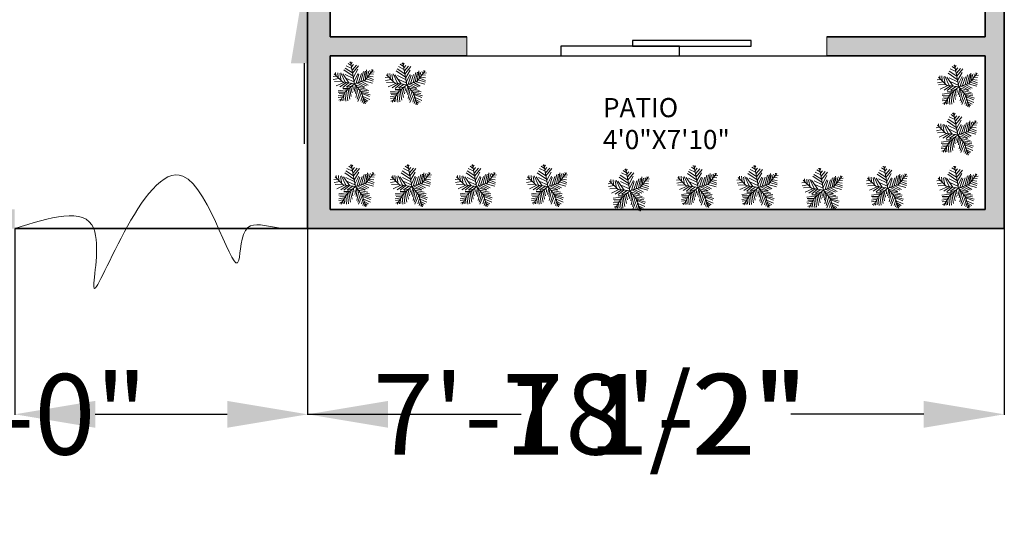
# Model space of a CAD drawing. Units: inches. Extents: x 35 to 5908, y 4 to 3165.
# Tile 2 of 6: x 5173 to 5481, y 2226 to 2387. Entities that reach past the tile are written whole.
import ezdxf

# ---------------------------------------------------------------- set-up
doc = ezdxf.new("R2010")
doc.units = ezdxf.units.IN
doc.header["$MEASUREMENT"] = 0
doc.linetypes.add('ACAD_ISO02W100', pattern=[15, 12, -3])
for name, color, linetype, lineweight in [('A-ANNO-DIMS', 2, 'Continuous', 18), ('A-ANNO-SYMB', 7, 'Continuous', 18), ('A-DOOR', 4, 'Continuous', 25), ('A-DOOR-HIDN', 4, 'ACAD_ISO02W100', 13), ('A-WALL', 7, 'Continuous', 35), ('A-WALL-PATT', 252, 'Continuous', 13), ('L-PLNT', 3, 'Continuous', 13)]:
    doc.layers.add(name, color=color, linetype=linetype, lineweight=lineweight)
doc.layers.add('A-AREA-IDEN', color=30, linetype='Continuous', lineweight=18, true_color=0xf8991e)
doc.styles.get("Standard").update_dxf_attribs({"font": 'arial.ttf'})
doc.dimstyles.get("Standard").update_dxf_attribs({"dimtxt": 25.18, "dimasz": 25.18, "dimexe": 0.18, "dimexo": 0.0625, "dimgap": 0.09, "dimtad": 0, "dimtih": 1, "dimtoh": 1, "dimdec": 0, "dimzin": 0, "dimdsep": 46, "dimlunit": 3, "dimtxsty": 'Standard', "dimcen": 0.09, "dimadec": 0, "dimazin": 0, "dimtfac": 1, "dimtdec": 0, "dimtofl": 0, "dimtmove": 0, "dimatfit": 3, "dimfxl": 1, "dimtolj": 1, "dimtzin": 0, "dimarcsym": 0})

# ---------------------------------------------------------------- blocks, each defined once
blk = doc.blocks.new('*U2')
for p, q in [((-8.737, 47.138), (-17.069, 52.711)), ((-10.186, 53.64), (-13.084, 55.962)), ((0, 0), (-10.5, 57)), ((-9.099, 51.782), (-6.563, 55.962)), ((-31.5, 4.5), (-52.5, 25.5)), ((-48.585, 21.131), (-49.309, 29.026)), ((-43.513, 28.561), (-42.427, 15.558)), ((-38.442, 26.239), (-34.819, 7.663)), ((-35.544, 28.097), (-24.314, 3.947)), ((-3.665, 19.273), (-27.574, 35.527)), ((-5.114, 28.097), (-24.676, 40.636)), ((-7.288, 39.707), (-21.778, 46.673)), ((-7.65, 43.423), (-2.578, 49.46)), ((-5.839, 35.992), (4.667, 48.067)), ((-5.114, 27.632), (10.463, 46.673)), ((-2.941, 16.486), (8.652, 37.85)), ((-1.129, 6.734), (9.014, 26.704)), ((10.101, 3.483), (17.708, 26.239)), ((16.259, 5.805), (23.142, 31.348)), ((22.055, 7.198), (27.489, 32.277)), ((27, 9), (48, 36)), ((27.127, 9.056), (31.112, 35.992)), ((31.836, 30.883), (32.561, 16.486)), ((35.096, 32.741), (37.27, 22.524)), ((38.719, 34.134), (41.979, 28.561)), ((40.53, 25.775), (48.862, 24.846)), ((43.791, 29.954), (51.036, 30.883)), ((44.153, 36.456), (45.239, 32.741)), ((-47.498, 19.737), (-55.83, 18.344)), ((-40.615, 13.7), (-55.105, 10.913)), ((-33.37, 6.269), (-52.207, 5.34)), ((-28.299, 3.483), (-47.86, -5.805)), ((-21.416, 3.018), (-38.079, -8.128)), ((0, 0), (-31.5, 4.5)), ((-14.533, 2.09), (-30.834, 25.31)), ((-15.982, 2.09), (-30.11, -9.521)), ((-24.314, 23.917), (-2.941, 13.7)), ((0, 0), (-22.5, -19.5)), ((-6.563, 1.161), (-21.416, -8.128)), ((-20.691, 13.7), (-1.129, 4.876)), ((0, 0), (27, 9)), ((0, 0), (18, -22.5)), ((3.942, 1.625), (11.187, 24.381)), ((6.478, 1.625), (26.04, -8.592)), ((11.187, 3.483), (30.749, -5.805)), ((18.07, 5.805), (35.096, -3.483)), ((24.229, 7.663), (46.688, 1.625)), ((29.662, 12.307), (48.137, 6.269)), ((33.285, 16.486), (48.862, 10.913)), ((36.183, 19.737), (48.137, 17.88)), ((-17.431, -15.094), (-42.789, -18.809)), ((-24.314, -21.596), (-42.427, -22.06)), ((-22.5, -19.5), (-37.5, -45)), ((-15.257, -12.772), (-30.11, -12.772)), ((-25.038, -23.918), (-22.865, -45.281)), ((-20.691, -18.345), (-17.793, -44.352)), ((-6.563, -5.805), (-19.967, -9.985)), ((-17.069, -15.094), (-12.721, -40.172)), ((-13.446, -11.378), (-8.737, -32.741)), ((-9.461, -8.592), (-6.201, -23.453)), ((-4.752, -3.483), (-3.665, -14.629)), ((2.493, -3.019), (-1.491, -20.202)), ((1.769, -2.555), (24.229, -9.521)), ((5.029, -6.27), (2.131, -25.775)), ((9.014, -11.378), (3.58, -35.992)), ((14.085, -16.951), (6.478, -40.172)), ((7.565, -9.056), (32.198, -14.629)), ((18.07, -22.524), (8.289, -45.745)), ((12.274, -15.094), (36.907, -18.809)), ((16.259, -19.738), (36.183, -22.989)), ((18, -22.5), (27, -52.5)), ((18.433, -22.524), (40.53, -29.026)), ((19.157, -25.311), (38.719, -33.206)), ((-28.299, -29.026), (-42.789, -31.348)), ((-30.834, -34.135), (-42.427, -35.528)), ((-34.457, -39.708), (-40.978, -42.494)), ((-26.849, -26.24), (-40.253, -25.775)), ((-32.646, -36.921), (-31.921, -44.352)), ((-29.023, -30.884), (-27.936, -43.887)), ((20.244, -30.419), (15.897, -44.816)), ((22.78, -37.85), (19.519, -48.532)), ((21.331, -32.741), (39.081, -40.636)), ((22.78, -38.314), (34.372, -44.816)), ((24.591, -45.745), (23.142, -50.854)), ((24.591, -43.423), (30.749, -47.603)), ((26.764, -49.925), (28.213, -50.854))]:
    blk.add_line(p, q)
blk = doc.blocks.new('*D26')
at = {"layer": 'A-ANNO-DIMS', "color": 0, "lineweight": -2, "transparency": 16777216}
for p, q in [((5241.11, 2433.5), (5215.93, 2433.5)), ((5266.29, 2429.02), (5266.29, 2433.68)), ((5296.57, 2429.02), (5296.57, 2433.68)), ((5321.75, 2433.5), (5346.93, 2433.5))]:
    blk.add_line(p, q, dxfattribs=at)
for points in [[(5241.11, 2437.7), (5241.11, 2429.3), (5266.29, 2433.5)], [(5321.75, 2437.7), (5321.75, 2429.3), (5296.57, 2433.5)]]:
    blk.add_solid(points, dxfattribs=at)
at = {"layer": 'Defpoints', "color": 0, "lineweight": -2, "transparency": 16777216}
for p in [(5266.29, 2433.5), (5266.29, 2428.96), (5296.57, 2428.96)]:
    blk.add_point(p, dxfattribs=at)
at = {"layer": 'A-ANNO-DIMS', "color": 0, "transparency": 16777216, "insert": (5025.37, 2433.5), "char_height": 25.18, "attachment_point": 5}
blk.add_mtext('\\A1;DOOR D1 2\'-6 1/2" TYP.', dxfattribs=at)
blk = doc.blocks.new('*D27')
at = {"layer": 'A-ANNO-DIMS', "color": 0, "lineweight": -2, "transparency": 16777216}
for p, q in [((5261.75, 2454.14), (5261.75, 2479.32)), ((5266.23, 2428.96), (5261.57, 2428.96)), ((5266.23, 2398.68), (5261.57, 2398.68)), ((5261.75, 2373.5), (5261.75, 2348.32))]:
    blk.add_line(p, q, dxfattribs=at)
for points in [[(5257.56, 2454.14), (5265.95, 2454.14), (5261.75, 2428.96)], [(5257.56, 2373.5), (5265.95, 2373.5), (5261.75, 2398.68)]]:
    blk.add_solid(points, dxfattribs=at)
at = {"layer": 'Defpoints', "color": 0, "lineweight": -2, "transparency": 16777216}
for p in [(5266.29, 2428.96), (5261.75, 2398.68), (5266.29, 2398.68)]:
    blk.add_point(p, dxfattribs=at)
at = {"layer": 'A-ANNO-DIMS', "color": 0, "transparency": 16777216, "insert": (5261.75, 2413.82), "char_height": 25.18, "attachment_point": 5}
blk.add_mtext('\\A1;2\'-6 1/2" TYP.', dxfattribs=at)
blk = doc.blocks.new('*D46')
at = {"layer": 'A-ANNO-DIMS', "color": 0, "lineweight": -2, "transparency": 16777216}
for p, q in [((5262.79, 2321.72), (5262.79, 2263.46)), ((5480.79, 2321.72), (5480.79, 2263.46)), ((5287.97, 2263.64), (5329.64, 2263.64)), ((5455.61, 2263.64), (5413.95, 2263.64))]:
    blk.add_line(p, q, dxfattribs=at)
for points in [[(5287.97, 2267.83), (5287.97, 2259.44), (5262.79, 2263.64)], [(5455.61, 2267.83), (5455.61, 2259.44), (5480.79, 2263.64)]]:
    blk.add_solid(points, dxfattribs=at)
at = {"layer": 'Defpoints', "color": 0, "lineweight": -2, "transparency": 16777216}
for p in [(5262.79, 2321.78), (5480.79, 2321.78), (5480.79, 2263.64)]:
    blk.add_point(p, dxfattribs=at)
at = {"layer": 'A-ANNO-DIMS', "color": 0, "transparency": 16777216, "insert": (5371.79, 2263.64), "char_height": 25.18, "attachment_point": 5}
blk.add_mtext('\\A1;18\'-2"', dxfattribs=at)
blk = doc.blocks.new('*D48')
at = {"layer": 'A-ANNO-DIMS', "color": 0, "lineweight": -2, "transparency": 16777216}
for p, q in [((5054.79, 2327.72), (5054.79, 2263.46)), ((5090.79, 2327.72), (5090.79, 2263.46)), ((5029.61, 2263.64), (5004.43, 2263.64)), ((5115.97, 2263.64), (5141.15, 2263.64))]:
    blk.add_line(p, q, dxfattribs=at)
for points in [[(5029.61, 2267.83), (5029.61, 2259.44), (5054.79, 2263.64)], [(5115.97, 2267.83), (5115.97, 2259.44), (5090.79, 2263.64)]]:
    blk.add_solid(points, dxfattribs=at)
at = {"layer": 'Defpoints', "color": 0, "lineweight": -2, "transparency": 16777216}
for p in [(5054.79, 2327.78), (5090.79, 2327.78), (5090.79, 2263.64)]:
    blk.add_point(p, dxfattribs=at)
at = {"layer": 'A-ANNO-DIMS', "color": 0, "transparency": 16777216, "insert": (5174.7, 2263.64), "char_height": 25.18, "attachment_point": 5}
blk.add_mtext('\\A1;3\'-0"', dxfattribs=at)
blk = doc.blocks.new('*D49')
at = {"layer": 'A-ANNO-DIMS', "color": 0, "lineweight": -2, "transparency": 16777216}
for p, q in [((5171.13, 2321.72), (5171.13, 2263.46)), ((5262.79, 2321.72), (5262.79, 2263.46)), ((5196.31, 2263.64), (5237.61, 2263.64)), ((5262.79, 2263.64), (5287.97, 2263.64))]:
    blk.add_line(p, q, dxfattribs=at)
for points in [[(5196.31, 2267.83), (5196.31, 2259.44), (5171.13, 2263.64)], [(5237.61, 2267.83), (5237.61, 2259.44), (5262.79, 2263.64)]]:
    blk.add_solid(points, dxfattribs=at)
at = {"layer": 'Defpoints', "color": 0, "lineweight": -2, "transparency": 16777216}
for p in [(5171.13, 2321.78), (5262.79, 2321.78), (5262.79, 2263.64)]:
    blk.add_point(p, dxfattribs=at)
at = {"layer": 'A-ANNO-DIMS', "color": 0, "transparency": 16777216, "insert": (5350.77, 2263.64), "char_height": 25.18, "attachment_point": 5}
blk.add_mtext('\\A1;7\'-7 1/2"', dxfattribs=at)

msp = doc.modelspace()

# ---------------------------------------------------------------- hatches: boundary and pattern name
at = {"layer": 'A-WALL-PATT'}
h = msp.add_hatch(color=256, dxfattribs=at)
h.dxf.hatch_style = 1
h.paths.add_polyline_path([(5198.29, 3041.78), (5119.29, 3041.78), (5119.29, 3035.78), (5155.79, 3035.78), (5155.79, 2967.78), (5087.79, 2967.78), (5087.79, 2966.78, -0.017236), (5087.79, 2964.78), (5087.79, 2961.78), (5262.79, 2961.78), (5262.79, 2967.78), (5236.55, 2967.78), (5236.55, 2967.75), (5218.53, 2967.75), (5161.79, 2967.78), (5161.79, 3035.78), (5198.29, 3035.78)])
h.paths.add_polyline_path([(5091.29, 3041.78), (5048.79, 3041.78), (5048.79, 2877.78), (5054.79, 2877.78), (5054.79, 2899), (5054.79, 2961.78), (5054.79, 2967.78), (5054.79, 3035.78), (5091.29, 3035.78)])
h.paths.add_polyline_path([(5346.29, 3041.78), (5226.29, 3041.78), (5226.29, 3035.78), (5262.79, 3035.78), (5269.79, 3035.78), (5346.29, 3035.78)])
h.paths.add_polyline_path([(5480.79, 3041.78), (5398.29, 3041.78), (5398.29, 3035.78), (5407.91, 3035.78), (5474.79, 3035.78), (5474.79, 2807.78), (5269.79, 2807.78), (5269.79, 3002.78), (5266.29, 3002.78, -0.017236), (5264.29, 3002.78), (5262.79, 3002.78), (5262.79, 2967.78), (5262.79, 2961.78), (5262.79, 2780.78), (5264.29, 2780.78, -0.014283), (5266.29, 2780.78), (5269.79, 2780.78), (5269.79, 2801.78), (5412.79, 2801.78), (5412.79, 2712.78), (5346.79, 2712.78), (5346.79, 2706.78), (5421.79, 2706.78), (5421.79, 2709.78, -0.017236), (5421.79, 2711.78), (5421.79, 2712.78), (5418.79, 2712.78), (5418.79, 2801.78), (5474.79, 2801.78), (5474.79, 2712.78), (5454.79, 2712.78), (5454.79, 2706.78), (5474.79, 2706.78), (5474.79, 2668.42), (5480.79, 2668.42)])
h.paths.add_polyline_path([(5054.79, 2825.78), (5048.79, 2825.78), (5048.79, 2632.28), (5054.79, 2632.28), (5054.79, 2642.69), (5054.79, 2735.78), (5262.79, 2735.78), (5262.79, 2741.78), (5054.79, 2741.78)])
h.paths.add_polyline_path([(5480.79, 2616.42), (5474.79, 2616.42), (5474.79, 2502.2), (5480.79, 2502.2)])
h.paths.add_polyline_path([(5407.53, 2562.78), (5269.79, 2562.78), (5269.79, 2696.78), (5266.29, 2696.78, -0.014283), (5264.29, 2696.78), (5262.79, 2696.78), (5262.79, 2509.78), (5264.29, 2509.78, -0.017236), (5266.29, 2509.78), (5269.79, 2509.78), (5269.79, 2556.78), (5407.53, 2556.78)])
h.paths.add_polyline_path([(5262.79, 2530.78), (5087.79, 2530.78), (5087.79, 2527.78, -0.017236), (5087.79, 2525.78), (5087.79, 2524.78), (5143.79, 2524.78), (5143.79, 2514.78), (5149.79, 2514.78), (5149.79, 2524.78), (5171.79, 2524.78), (5171.79, 2514.78), (5177.79, 2514.78), (5177.79, 2524.78), (5262.79, 2524.78)], flags=17)
h.paths.add_polyline_path([(5262.79, 2395.71), (5262.79, 2321.78), (5480.79, 2321.78), (5480.79, 2450.2), (5474.79, 2450.2), (5474.79, 2381.78), (5425.29, 2381.78), (5425.29, 2375.78), (5474.79, 2375.78), (5474.79, 2327.78), (5269.79, 2327.78), (5269.79, 2375.78), (5312.61, 2375.78), (5312.61, 2381.78), (5269.79, 2381.78), (5269.79, 2395.71)])
h.paths.add_polyline_path([(5171.13, 2321.78), (5171.13, 2327.78), (5054.79, 2327.78), (5054.79, 2470.78), (5157.79, 2470.78), (5262.79, 2470.78), (5262.79, 2461.71), (5269.79, 2461.71), (5269.79, 2476.78), (5262.79, 2476.78), (5177.79, 2476.78), (5177.79, 2486.78), (5171.79, 2486.78), (5171.79, 2476.78), (5149.79, 2476.78), (5149.79, 2486.78), (5143.79, 2486.78), (5143.79, 2476.78), (5054.79, 2476.78), (5054.79, 2580.28), (5048.79, 2580.28), (5048.79, 2321.78)])

# ---------------------------------------------------------------- linework, layer by layer
at = {"layer": 'A-ANNO-SYMB'}
msp.add_open_spline([(5171.13, 2321.78), (5182.06, 2325.26), (5201.09, 2331.32), (5190.06, 2279.32), (5222.38, 2375.47), (5241.98, 2295.8), (5241.68, 2325.16), (5253.78, 2321.34), (5259.7, 2321.63), (5262.79, 2321.78)], degree=3, knots=[0, 0, 0, 0, 24.730916, 43.022674, 87.561703, 119.186713, 129.816728, 138.741517, 148.526637, 148.526637, 148.526637, 148.526637], dxfattribs=at)
at = {"layer": 'A-DOOR'}
msp.add_line((5312.61, 2375.78), (5425.29, 2375.78), dxfattribs=at)
for points in [[(5342, 2375.78), (5379.2, 2375.78), (5379.2, 2378.89), (5342, 2378.89)], [(5364.5, 2378.89), (5401.61, 2378.89), (5401.61, 2380.61), (5364.5, 2380.61)]]:
    msp.add_lwpolyline(points, close=True, dxfattribs=at)
at = {"layer": 'A-DOOR-HIDN'}
for p, q in [((5312.61, 2381.78), (5312.61, 2375.78)), ((5425.29, 2381.78), (5425.29, 2375.78))]:
    msp.add_line(p, q, dxfattribs=at)
at = {"layer": 'A-WALL'}
for p, q in [((5480.79, 3041.78), (5480.79, 2321.78)), ((5474.79, 2706.78), (5474.79, 2381.78)), ((5269.79, 2400.68), (5269.79, 2381.78)), ((5262.79, 2327.78), (5262.79, 2398.71)), ((5312.61, 2381.78), (5269.79, 2381.78)), ((5474.79, 2381.78), (5425.29, 2381.78)), ((5269.79, 2375.78), (5269.79, 2327.78)), ((5312.61, 2375.78), (5269.79, 2375.78)), ((5474.79, 2375.78), (5425.29, 2375.78)), ((5474.79, 2375.78), (5474.79, 2327.78)), ((5262.79, 2327.78), (5262.79, 2321.78)), ((5474.79, 2327.78), (5269.79, 2327.78)), ((5171.13, 2321.78), (5262.79, 2321.78)), ((5480.79, 2321.78), (5262.79, 2321.78))]:
    msp.add_line(p, q, dxfattribs=at)

# ---------------------------------------------------------------- block references
at = {"layer": 'L-PLNT', "xscale": 0.1208865601236175, "yscale": 0.1208865601236175, "zscale": 0.1208865601236175}
for p in [(5277.49, 2367.1), (5293.81, 2366.79), (5466.53, 2366.08), (5466.21, 2351.08), (5277.73, 2334.89), (5295.38, 2334.89), (5315.68, 2334.89), (5337.98, 2334.89), (5363.62, 2333.56), (5384.95, 2334.66), (5403.85, 2334.66), (5424.22, 2333.82), (5444.38, 2334.45), (5466.43, 2334.45)]:
    msp.add_blockref('*U2', p, dxfattribs=at)

# ---------------------------------------------------------------- texts
at = {"layer": 'A-AREA-IDEN', "insert": (5355.2, 2362.62), "char_height": 6, "attachment_point": 1}
msp.add_mtext_dynamic_manual_height_columns('PATIO\\P4\'0"X7\'10"', width=69.8687, gutter_width=1, heights=[0], dxfattribs=at)

# ---------------------------------------------------------------- dimensions: what is measured, and where the dimension line sits
at = {"layer": 'A-ANNO-DIMS'}
for base, p1, p2, angle, text, picture, middle in [((5266.29, 2433.5), (5296.57, 2428.96), (5266.29, 2428.96), 180, 'DOOR D1 <> TYP.', '*D26', (5025.37, 2433.5)), ((5261.75, 2398.68), (5266.29, 2428.96), (5266.29, 2398.68), 270, '<> TYP.', '*D27', (5261.75, 2413.82))]:
    dim = msp.add_linear_dim(base=base, p1=p1, p2=p2, angle=angle, text=text, dimstyle='Standard', override={"dimdec": 1, "dimlfac": 1, "dimrnd": 0, "dimzin": 1, "dimdsep": 46, "dimlunit": 4, "dimfrac": 2}, dxfattribs=at)
    dim.commit()
    dim.dimension.update_dxf_attribs({"geometry": picture, "text_midpoint": middle})
for base, p1, p2, picture, middle in [((5090.79, 2263.64), (5054.79, 2327.78), (5090.79, 2327.78), '*D48', (5174.7, 2263.64)), ((5262.79, 2263.64), (5171.13, 2321.78), (5262.79, 2321.78), '*D49', (5350.77, 2263.64)), ((5480.79, 2263.64), (5262.79, 2321.78), (5480.79, 2321.78), '*D46', (5371.79, 2263.64))]:
    dim = msp.add_linear_dim(base=base, p1=p1, p2=p2, dimstyle='Standard', override={"dimdec": 1, "dimlfac": 1, "dimrnd": 0, "dimzin": 1, "dimdsep": 46, "dimlunit": 4, "dimfrac": 2}, dxfattribs=at)
    dim.commit()
    dim.dimension.update_dxf_attribs({"geometry": picture, "text_midpoint": middle})

doc.saveas('drawing.dxf')
